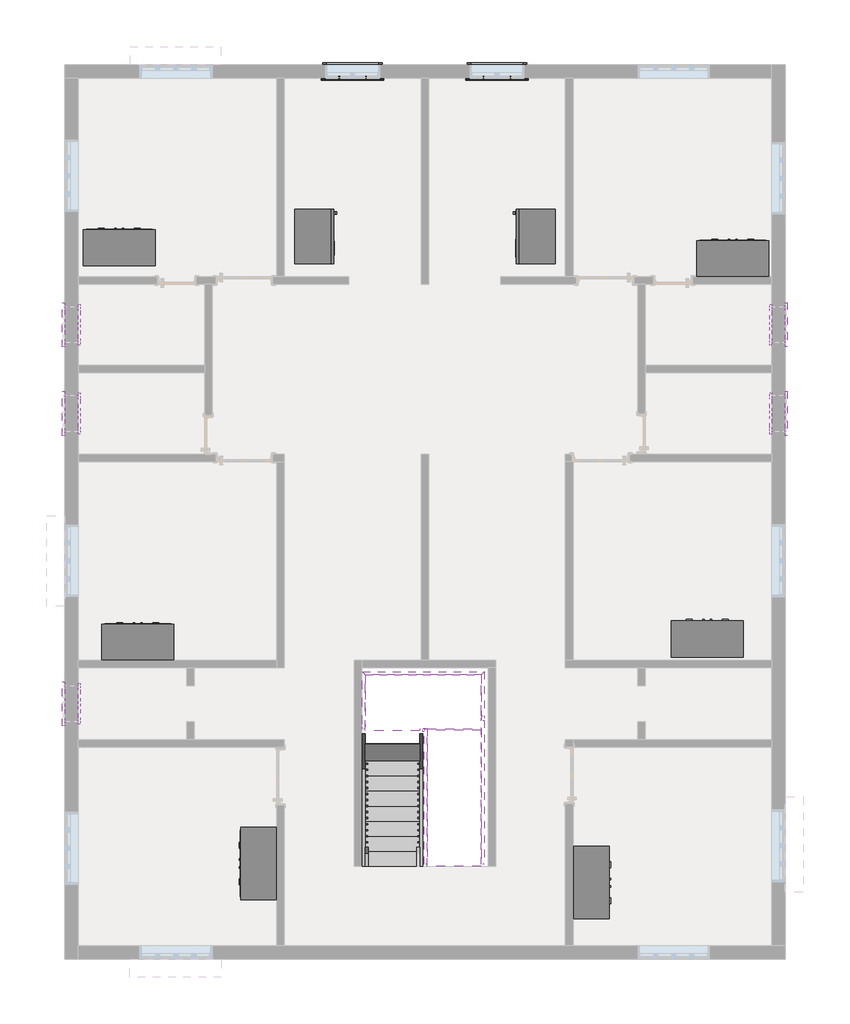
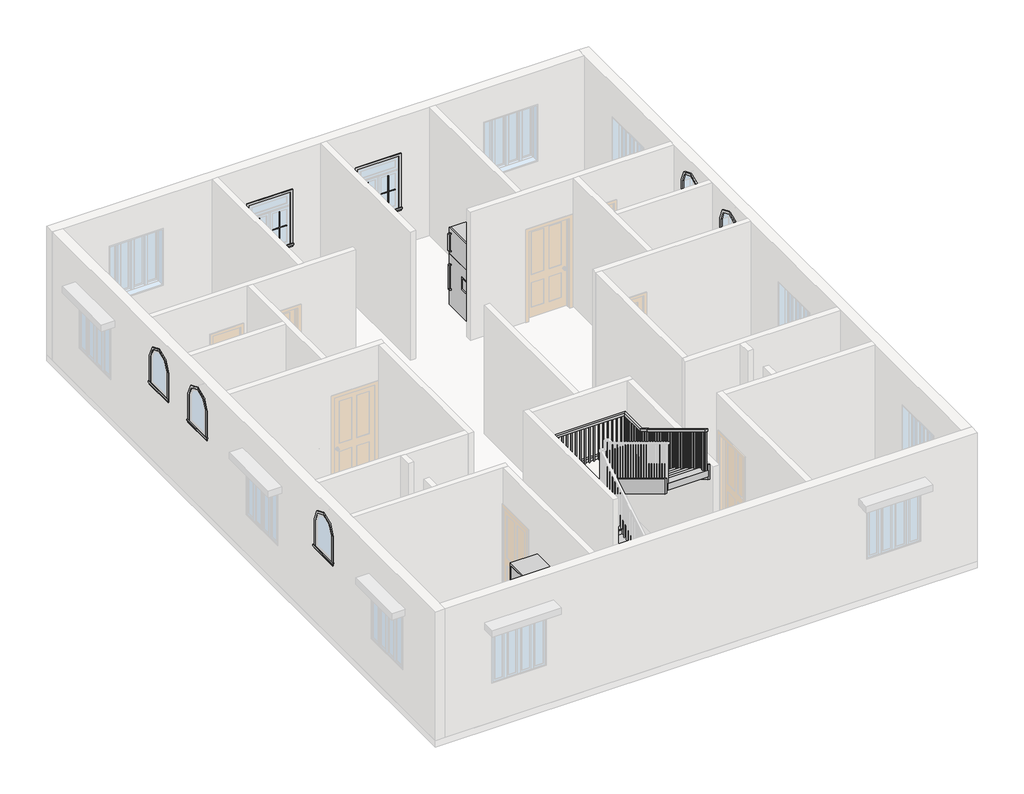
# One storey, part 3 of 4: 18 proxies, 8 furniture elements, 8 members, 2 stair flights, 1 railing, 1 slab.
"""IFC4 building model written with IfcOpenShell, lengths in millimetres."""

from ifc_helpers import new_model, si_unit, frame, origin, place, context, project, spatial, polyline, outline, extrude, faceted_brep, transform, mapped, element, save
from components import muntin_pattern_2x2_muntin_pattern_2x2_d1c6e638, muntin_pattern_2x2_muntin_pattern_2x2_37b95fb2, trim_window_exterior_flat_with_sill_80371c4b, trim_window_exterior_flat_arch_top_tree_centered_with_sill_b3d54518, trim_window_interior_flat_picture_frame_c1dcbb6d, trim_window_interior_flat_arch_top_tree_centered_picture_1d59b3d4, furniture_65fa61b5, furniture_3f4f9d7a, furniture_82e269c4, non_monolithic_landing_0f5a95a9, stair_flight_63be9a33, stair_flight_b6fb1fe0

model = new_model("IFC4")

# Units and contexts
model_context = context("Model", 3, world=origin())
ifc_project = project(units=[si_unit("LENGTHUNIT", "METRE", prefix="MILLI")], contexts=[model_context])

# Site, building, storey
site = spatial("IfcSite", under=ifc_project)
building = spatial("IfcBuilding", under=site)
storey = spatial("IfcBuildingStorey", under=building, Elevation=3352.8)

# Proxies
placement = place(None, origin())
muntin_pattern_2x2_muntin_pattern_2x2_shape = muntin_pattern_2x2_muntin_pattern_2x2_d1c6e638(model_context)
element("IfcBuildingElementProxy", 1, Name="Muntin Pattern_2x2 : Muntin Pattern_2x2", ObjectType="Muntin Pattern_2x2 : Muntin Pattern_2x2", at=placement, inside=storey, context=model_context, shape_type="MappedRepresentation", body=[
    mapped(muntin_pattern_2x2_muntin_pattern_2x2_shape, transform((-10531.1646954, 8361.6522103, 4337.05), x_axis=(-1.0, 0.0, 0.0), y_axis=(0.0, -1.0, 0.0), z_axis=(0.0, 0.0, 1.0))),
])
element("IfcBuildingElementProxy", 2, Name="Muntin Pattern_2x2 : Muntin Pattern_2x2", ObjectType="Muntin Pattern_2x2 : Muntin Pattern_2x2", at=placement, inside=storey, context=model_context, shape_type="MappedRepresentation", body=[
    mapped(muntin_pattern_2x2_muntin_pattern_2x2_shape, transform((-8092.7646954, 8361.6522103, 4337.05), x_axis=(-1.0, 0.0, 0.0), y_axis=(0.0, -1.0, 0.0), z_axis=(0.0, 0.0, 1.0))),
])
muntin_pattern_2x2_muntin_pattern_2x2_2_shape = muntin_pattern_2x2_muntin_pattern_2x2_37b95fb2(model_context)
element("IfcBuildingElementProxy", 3, Name="Muntin Pattern_2x2 : Muntin Pattern_2x2", ObjectType="Muntin Pattern_2x2 : Muntin Pattern_2x2", at=placement, inside=storey, context=model_context, shape_type="MappedRepresentation", body=[
    mapped(muntin_pattern_2x2_muntin_pattern_2x2_2_shape, transform((-10985.1896954, 8361.6522103, 4337.05), x_axis=(1.0, 0.0, 0.0), y_axis=(0.0, 1.0, 0.0), z_axis=(0.0, 0.0, 1.0))),
])
element("IfcBuildingElementProxy", 4, Name="Muntin Pattern_2x2 : Muntin Pattern_2x2", ObjectType="Muntin Pattern_2x2 : Muntin Pattern_2x2", at=placement, inside=storey, context=model_context, shape_type="MappedRepresentation", body=[
    mapped(muntin_pattern_2x2_muntin_pattern_2x2_2_shape, transform((-8546.7896954, 8361.6522103, 4337.05), x_axis=(1.0, 0.0, 0.0), y_axis=(0.0, 1.0, 0.0), z_axis=(0.0, 0.0, 1.0))),
])
trim_window_exterior_flat_with_sill_shape = trim_window_exterior_flat_with_sill_80371c4b(model_context)
element("IfcBuildingElementProxy", 5, Name="Trim-Window-Exterior-Flat : with Sill", ObjectType="Trim-Window-Exterior-Flat : with Sill", at=placement, inside=storey, context=model_context, shape_type="MappedRepresentation", body=[
    mapped(trim_window_exterior_flat_with_sill_shape, transform((-10758.1771954, 8352.1272103, 5486.4), x_axis=(-1.0, 0.0, 0.0), y_axis=(0.0, 0.0, -1.0), z_axis=(0.0, -1.0, 0.0))),
])
element("IfcBuildingElementProxy", 6, Name="Trim-Window-Exterior-Flat : with Sill", ObjectType="Trim-Window-Exterior-Flat : with Sill", at=placement, inside=storey, context=model_context, shape_type="MappedRepresentation", body=[
    mapped(trim_window_exterior_flat_with_sill_shape, transform((-8319.7771954, 8352.1272103, 5486.4), x_axis=(-1.0, 0.0, 0.0), y_axis=(0.0, 0.0, -1.0), z_axis=(0.0, -1.0, 0.0))),
])
trim_window_exterior_flat_arch_top_tree_centered_with_sill_shape = trim_window_exterior_flat_arch_top_tree_centered_with_sill_b3d54518(model_context)
element("IfcBuildingElementProxy", 7, Name="Trim-Window-Exterior-Flat-Arch-Top-Tree_Centered : with Sill", ObjectType="Trim-Window-Exterior-Flat-Arch-Top-Tree_Centered : with Sill", at=placement, inside=storey, context=model_context, shape_type="MappedRepresentation", body=[
    mapped(trim_window_exterior_flat_arch_top_tree_centered_with_sill_shape, transform((-15623.8646954, -2214.2727897, 6096.0), x_axis=(0.0, -1.0, 0.0), y_axis=(0.0, 0.0, 1.0), z_axis=(-1.0, 0.0, 0.0))),
])
element("IfcBuildingElementProxy", 8, Name="Trim-Window-Exterior-Flat-Arch-Top-Tree_Centered : with Sill", ObjectType="Trim-Window-Exterior-Flat-Arch-Top-Tree_Centered : with Sill", at=placement, inside=storey, context=model_context, shape_type="MappedRepresentation", body=[
    mapped(trim_window_exterior_flat_arch_top_tree_centered_with_sill_shape, transform((-3455.6771954, 2688.1919086, 6096.0), x_axis=(0.0, 1.0, 0.0), y_axis=(0.0, 0.0, 1.0), z_axis=(1.0, 0.0, 0.0))),
])
element("IfcBuildingElementProxy", 9, Name="Trim-Window-Exterior-Flat-Arch-Top-Tree_Centered : with Sill", ObjectType="Trim-Window-Exterior-Flat-Arch-Top-Tree_Centered : with Sill", at=placement, inside=storey, context=model_context, shape_type="MappedRepresentation", body=[
    mapped(trim_window_exterior_flat_arch_top_tree_centered_with_sill_shape, transform((-3455.6771954, 4186.5272103, 6096.0), x_axis=(0.0, 1.0, 0.0), y_axis=(0.0, 0.0, 1.0), z_axis=(1.0, 0.0, 0.0))),
])
element("IfcBuildingElementProxy", 10, Name="Trim-Window-Exterior-Flat-Arch-Top-Tree_Centered : with Sill", ObjectType="Trim-Window-Exterior-Flat-Arch-Top-Tree_Centered : with Sill", at=placement, inside=storey, context=model_context, shape_type="MappedRepresentation", body=[
    mapped(trim_window_exterior_flat_arch_top_tree_centered_with_sill_shape, transform((-15623.8646954, 2688.1919086, 6096.0), x_axis=(0.0, -1.0, 0.0), y_axis=(0.0, 0.0, 1.0), z_axis=(-1.0, 0.0, 0.0))),
])
element("IfcBuildingElementProxy", 11, Name="Trim-Window-Exterior-Flat-Arch-Top-Tree_Centered : with Sill", ObjectType="Trim-Window-Exterior-Flat-Arch-Top-Tree_Centered : with Sill", at=placement, inside=storey, context=model_context, shape_type="MappedRepresentation", body=[
    mapped(trim_window_exterior_flat_arch_top_tree_centered_with_sill_shape, transform((-15623.8646954, 4186.5272103, 6096.0), x_axis=(0.0, -1.0, 0.0), y_axis=(0.0, 0.0, 1.0), z_axis=(-1.0, 0.0, 0.0))),
])
trim_window_interior_flat_picture_frame_shape = trim_window_interior_flat_picture_frame_c1dcbb6d(model_context)
element("IfcBuildingElementProxy", 12, Name="Trim-Window-Interior-Flat : Picture Frame", ObjectType="Trim-Window-Interior-Flat : Picture Frame", at=placement, inside=storey, context=model_context, shape_type="MappedRepresentation", body=[
    mapped(trim_window_interior_flat_picture_frame_shape, transform((-10758.1771954, 8580.7272103, 5486.4), x_axis=(1.0, 0.0, 0.0), y_axis=(0.0, 0.0, -1.0), z_axis=(0.0, 1.0, 0.0))),
])
element("IfcBuildingElementProxy", 13, Name="Trim-Window-Interior-Flat : Picture Frame", ObjectType="Trim-Window-Interior-Flat : Picture Frame", at=placement, inside=storey, context=model_context, shape_type="MappedRepresentation", body=[
    mapped(trim_window_interior_flat_picture_frame_shape, transform((-8319.7771954, 8580.7272103, 5486.4), x_axis=(1.0, 0.0, 0.0), y_axis=(0.0, 0.0, -1.0), z_axis=(0.0, 1.0, 0.0))),
])
trim_window_interior_flat_arch_top_tree_centered_picture_shape = trim_window_interior_flat_arch_top_tree_centered_picture_1d59b3d4(model_context)
element("IfcBuildingElementProxy", 14, Name="Trim-Window-Interior-Flat-Arch-Top-Tree_Centered : Picture Frame", ObjectType="Trim-Window-Interior-Flat-Arch-Top-Tree_Centered : Picture Frame", at=placement, inside=storey, context=model_context, shape_type="MappedRepresentation", body=[
    mapped(trim_window_interior_flat_arch_top_tree_centered_picture_shape, transform((-15395.2646954, -2214.2727897, 6096.0), x_axis=(0.0, 1.0, 0.0), y_axis=(0.0, 0.0, 1.0), z_axis=(1.0, 0.0, 0.0))),
])
element("IfcBuildingElementProxy", 15, Name="Trim-Window-Interior-Flat-Arch-Top-Tree_Centered : Picture Frame", ObjectType="Trim-Window-Interior-Flat-Arch-Top-Tree_Centered : Picture Frame", at=placement, inside=storey, context=model_context, shape_type="MappedRepresentation", body=[
    mapped(trim_window_interior_flat_arch_top_tree_centered_picture_shape, transform((-3684.2771954, 2688.1919086, 6096.0), x_axis=(0.0, -1.0, 0.0), y_axis=(0.0, 0.0, 1.0), z_axis=(-1.0, 0.0, 0.0))),
])
element("IfcBuildingElementProxy", 16, Name="Trim-Window-Interior-Flat-Arch-Top-Tree_Centered : Picture Frame", ObjectType="Trim-Window-Interior-Flat-Arch-Top-Tree_Centered : Picture Frame", at=placement, inside=storey, context=model_context, shape_type="MappedRepresentation", body=[
    mapped(trim_window_interior_flat_arch_top_tree_centered_picture_shape, transform((-3684.2771954, 4186.5272103, 6096.0), x_axis=(0.0, -1.0, 0.0), y_axis=(0.0, 0.0, 1.0), z_axis=(-1.0, 0.0, 0.0))),
])
element("IfcBuildingElementProxy", 17, Name="Trim-Window-Interior-Flat-Arch-Top-Tree_Centered : Picture Frame", ObjectType="Trim-Window-Interior-Flat-Arch-Top-Tree_Centered : Picture Frame", at=placement, inside=storey, context=model_context, shape_type="MappedRepresentation", body=[
    mapped(trim_window_interior_flat_arch_top_tree_centered_picture_shape, transform((-15395.2646954, 2688.1919086, 6096.0), x_axis=(0.0, 1.0, 0.0), y_axis=(0.0, 0.0, 1.0), z_axis=(1.0, 0.0, 0.0))),
])
element("IfcBuildingElementProxy", 18, Name="Trim-Window-Interior-Flat-Arch-Top-Tree_Centered : Picture Frame", ObjectType="Trim-Window-Interior-Flat-Arch-Top-Tree_Centered : Picture Frame", at=placement, inside=storey, context=model_context, shape_type="MappedRepresentation", body=[
    mapped(trim_window_interior_flat_arch_top_tree_centered_picture_shape, transform((-15395.2646954, 4186.5272103, 6096.0), x_axis=(0.0, 1.0, 0.0), y_axis=(0.0, 0.0, 1.0), z_axis=(1.0, 0.0, 0.0))),
])

# Furniture
furniture_shape = furniture_65fa61b5(model_context)
element("IfcFurniture", 19, at=placement, inside=storey, context=model_context, shape_type="MappedRepresentation", body=[
    mapped(furniture_shape, transform((-11740.80602, 6289.078474, 3352.8), x_axis=(0.0, 1.0, 0.0), y_axis=(-1.0, 0.0, 0.0), z_axis=(0.0, 0.0, 1.0))),
])
furniture_2_shape = furniture_3f4f9d7a(model_context)
element("IfcFurniture", 20, at=placement, inside=storey, context=model_context, shape_type="MappedRepresentation", body=[
    mapped(furniture_2_shape, transform((-7338.7358708, 6289.078474, 3352.8), x_axis=(0.0, 1.0, 0.0), y_axis=(-1.0, 0.0, 0.0), z_axis=(0.0, 0.0, 1.0))),
])
furniture_3_shape = furniture_82e269c4(model_context)
element("IfcFurniture", 21, ObjectType="Wardrobe : 48\" x 72\" x 24\"", at=placement, inside=storey, context=model_context, shape_type="MappedRepresentation", body=[
    mapped(furniture_3_shape, transform((-14969.1544857, 4905.0525787, 3352.8), x_axis=(-1.0, 0.0, 0.0), y_axis=(0.0, -1.0, 0.0), z_axis=(0.0, 0.0, 1.0))),
])
element("IfcFurniture", 22, ObjectType="Wardrobe : 48\" x 72\" x 24\"", at=placement, inside=storey, context=model_context, shape_type="MappedRepresentation", body=[
    mapped(furniture_3_shape, transform((-4609.4240791, 4720.3884008, 3352.8), x_axis=(-1.0, 0.0, 0.0), y_axis=(0.0, -1.0, 0.0), z_axis=(0.0, 0.0, 1.0))),
])
element("IfcFurniture", 23, ObjectType="Wardrobe : 48\" x 72\" x 24\"", at=placement, inside=storey, context=model_context, shape_type="MappedRepresentation", body=[
    mapped(furniture_3_shape, transform((-14654.9354475, -1756.6115992, 3352.8), x_axis=(-1.0, 0.0, 0.0), y_axis=(0.0, -1.0, 0.0), z_axis=(0.0, 0.0, 1.0))),
])
element("IfcFurniture", 24, ObjectType="Wardrobe : 48\" x 72\" x 24\"", at=placement, inside=storey, context=model_context, shape_type="MappedRepresentation", body=[
    mapped(furniture_3_shape, transform((-5037.6875981, -1704.33178, 3352.8), x_axis=(-1.0, 0.0, 0.0), y_axis=(0.0, -1.0, 0.0), z_axis=(0.0, 0.0, 1.0))),
])
element("IfcFurniture", 25, ObjectType="Wardrobe : 48\" x 72\" x 24\"", at=placement, inside=storey, context=model_context, shape_type="MappedRepresentation", body=[
    mapped(furniture_3_shape, transform((-7316.016005, -4965.0574511, 3352.8), x_axis=(0.0, 1.0, 0.0), y_axis=(-1.0, 0.0, 0.0), z_axis=(0.0, 0.0, 1.0))),
])
element("IfcFurniture", 26, ObjectType="Wardrobe : 48\" x 72\" x 24\"", at=placement, inside=storey, context=model_context, shape_type="MappedRepresentation", body=[
    mapped(furniture_3_shape, transform((-11761.9383858, -5181.4279362, 3352.8), x_axis=(0.0, -1.0, 0.0), y_axis=(1.0, 0.0, 0.0), z_axis=(0.0, 0.0, 1.0))),
])

# Members
element("IfcMember", 27, ObjectType="Stringer - 2\" Width", at=placement, inside=storey, context=model_context, shape_type="SweptSolid", body=[
    extrude(outline(polyline([(-4957.4727897, 3352.8), (-4957.4727897, 3564.3517384), (-2643.0590204, 4953.0), (-2558.6343079, 4648.2), (-4717.6343079, 3352.8), (-4957.4727897, 3352.8)])), frame((-10593.0771954, 0.0, 0.0), z_axis=(1.0, 0.0, 0.0), x_axis=(0.0, 1.0, 0.0)), (0.0, 0.0, 1.0), 50.8),
])
element("IfcMember", 28, ObjectType="Stringer - 2\" Width", at=placement, inside=storey, context=model_context, shape_type="SweptSolid", body=[
    extrude(outline(polyline([(-4957.4727897, 3352.8), (-4957.4727897, 3564.3517384), (-2643.0590204, 4953.0), (-2639.7227897, 4953.0), (-2639.7227897, 4599.5469109), (-4717.6343079, 3352.8), (-4957.4727897, 3352.8)])), frame((-9627.8771954, 0.0, 0.0), z_axis=(1.0, 0.0, 0.0), x_axis=(0.0, 1.0, 0.0)), (0.0, 0.0, 1.0), 50.8),
])
element("IfcMember", 29, ObjectType="Stringer - 2\" Width", at=placement, inside=storey, context=model_context, shape_type="SweptSolid", body=[
    extrude(outline(polyline([(-2414.1365589, 4953.0), (-2498.5612714, 4648.2), (-4925.7227897, 6104.4969109), (-4925.7227897, 6459.9517384), (-2414.1365589, 4953.0)])), frame((-8586.4771954, 0.0, 0.0), z_axis=(1.0, 0.0, 0.0), x_axis=(0.0, 1.0, 0.0)), (0.0, 0.0, 1.0), 50.8),
])
element("IfcMember", 30, ObjectType="Stringer - 2\" Width", at=placement, inside=storey, context=model_context, shape_type="SweptSolid", body=[
    extrude(outline(polyline([(-2639.7227897, 5088.3517384), (-2639.7227897, 4732.8969109), (-4925.7227897, 6104.4969109), (-4925.7227897, 6459.9517384), (-2639.7227897, 5088.3517384)])), frame((-9551.6771954, 0.0, 0.0), z_axis=(1.0, 0.0, 0.0), x_axis=(0.0, 1.0, 0.0)), (0.0, 0.0, 1.0), 50.8),
])
element("IfcMember", 31, ObjectType="Stringer - 2\" Width", at=placement, inside=storey, context=model_context, shape_type="Brep", body=[
    faceted_brep([(-8586.4771954, -2414.1365589, 4953.0), (-8535.6771954, -2414.1365589, 4953.0), (-8535.6771954, -1674.5227897, 4953.0), (-8586.4771954, -1725.3227897, 4953.0), (-8586.4771954, -2498.5612714, 4648.2), (-8586.4771954, -1725.3227897, 4648.2), (-8535.6771954, -2498.5612714, 4648.2), (-8535.6771954, -1674.5227897, 4648.2)], [[[0, 1, 2, 3]], [[4, 0, 3, 5]], [[6, 4, 5, 7]], [[1, 6, 7, 2]], [[1, 0, 4, 6]], [[2, 7, 5, 3]]]),
])
element("IfcMember", 32, ObjectType="Stringer - 2\" Width", at=placement, inside=storey, context=model_context, shape_type="SweptSolid", body=[
    extrude(outline(polyline([(-8535.6771954, -1674.5227897), (-8586.4771954, -1725.3227897), (-10542.2771954, -1725.3227897), (-10593.0771954, -1674.5227897), (-8535.6771954, -1674.5227897)])), frame((0.0, 0.0, 4648.2), z_axis=(0.0, 0.0, 1.0), x_axis=(1.0, 0.0, 0.0)), (0.0, 0.0, 1.0), 304.8),
])
element("IfcMember", 33, ObjectType="Stringer - 2\" Width", at=placement, inside=storey, context=model_context, shape_type="Brep", body=[
    faceted_brep([(-10542.2771954, -1725.3227897, 4953.0), (-10593.0771954, -1674.5227897, 4953.0), (-10593.0771954, -2643.0590204, 4953.0), (-10542.2771954, -2643.0590204, 4953.0), (-10542.2771954, -1725.3227897, 4648.2), (-10542.2771954, -2558.6343079, 4648.2), (-10593.0771954, -1674.5227897, 4648.2), (-10593.0771954, -2558.6343079, 4648.2)], [[[0, 1, 2, 3]], [[4, 0, 3, 5]], [[6, 4, 5, 7]], [[1, 6, 7, 2]], [[1, 0, 4, 6]], [[2, 7, 5, 3]]]),
])
element("IfcMember", 34, ObjectType="Stringer - 2\" Width", at=placement, inside=storey, context=model_context, shape_type="SweptSolid", body=[
    extrude(outline(polyline([(-9577.0771954, -2690.5227897), (-9577.0771954, -2639.7227897), (-9551.6771954, -2639.7227897), (-9551.6771954, -2690.5227897), (-9577.0771954, -2690.5227897)])), frame((0.0, 0.0, 4648.2), z_axis=(0.0, 0.0, 1.0), x_axis=(1.0, 0.0, 0.0)), (0.0, 0.0, 1.0), 304.8),
])

# Railing
element("IfcRailing", 35, ObjectType="Handrail - Rectangular", at=placement, inside=storey, context=model_context, shape_type="SolidModel", body=[
    faceted_brep([(-10542.2771954, -4957.4727897, 4419.6), (-10542.2771954, -4957.4727897, 4360.3575287), (-10491.4771954, -4957.4727897, 4360.3575287), (-10491.4771954, -4957.4727897, 4419.6), (-10542.2771954, -2671.4727897, 5791.2), (-10542.2771954, -2657.4020042, 5740.4), (-10491.4771954, -2657.4020042, 5740.4), (-10491.4771954, -2671.4727897, 5791.2), (-10542.2771954, -1725.3227897, 5791.2), (-10542.2771954, -1725.3227897, 5740.4), (-10491.4771954, -1776.1227897, 5740.4), (-10491.4771954, -1776.1227897, 5791.2), (-8586.4771954, -1725.3227897, 5791.2), (-8586.4771954, -1725.3227897, 5740.4), (-8637.2771954, -1776.1227897, 5740.4), (-8637.2771954, -1776.1227897, 5791.2), (-8586.4771954, -2385.7227897, 5791.2), (-8586.4771954, -2399.7935751, 5740.4), (-8637.2771954, -2399.7935751, 5740.4), (-8637.2771954, -2385.7227897, 5791.2), (-8586.4771954, -2639.7227897, 5943.6), (-8586.4771954, -2665.859174, 5900.0393594), (-8637.2771954, -2665.859174, 5900.0393594), (-8637.2771954, -2639.7227897, 5943.6), (-8586.4771954, -4925.7227897, 7315.2), (-8637.2771954, -4925.7227897, 7315.2), (-8637.2771954, -4925.7227897, 7255.9575287), (-8586.4771954, -4925.7227897, 7255.9575287)], [[[0, 1, 2, 3]], [[1, 0, 4, 5]], [[2, 1, 5, 6]], [[3, 2, 6, 7]], [[0, 3, 7, 4]], [[5, 4, 8, 9]], [[6, 5, 9, 10]], [[7, 6, 10, 11]], [[4, 7, 11, 8]], [[9, 8, 12, 13]], [[10, 9, 13, 14]], [[11, 10, 14, 15]], [[8, 11, 15, 12]], [[13, 12, 16, 17]], [[14, 13, 17, 18]], [[15, 14, 18, 19]], [[12, 15, 19, 16]], [[17, 16, 20, 21]], [[18, 17, 21, 22]], [[19, 18, 22, 23]], [[16, 19, 23, 20]], [[24, 25, 26, 27]], [[21, 20, 24, 27]], [[22, 21, 27, 26]], [[23, 22, 26, 25]], [[20, 23, 25, 24]]]),
    extrude(outline(polyline([(-4865.3977897, 7219.7625287), (-4865.3977897, 6248.4), (-4884.4477897, 6248.4), (-4884.4477897, 7231.1925287), (-4865.3977897, 7219.7625287)])), frame((-8621.4021954, 0.0, 0.0), z_axis=(1.0, 0.0, 0.0), x_axis=(0.0, 1.0, 0.0)), (0.0, 0.0, 1.0), 19.05),
    extrude(outline(polyline([(-4763.7977897, 7158.8025287), (-4763.7977897, 6248.4), (-4782.8477897, 6248.4), (-4782.8477897, 7170.2325287), (-4763.7977897, 7158.8025287)])), frame((-8621.4021954, 0.0, 0.0), z_axis=(1.0, 0.0, 0.0), x_axis=(0.0, 1.0, 0.0)), (0.0, 0.0, 1.0), 19.05),
    extrude(outline(polyline([(-4662.1977897, 7097.8425287), (-4662.1977897, 6248.4), (-4681.2477897, 6248.4), (-4681.2477897, 7109.2725287), (-4662.1977897, 7097.8425287)])), frame((-8621.4021954, 0.0, 0.0), z_axis=(1.0, 0.0, 0.0), x_axis=(0.0, 1.0, 0.0)), (0.0, 0.0, 1.0), 19.05),
    extrude(outline(polyline([(-4560.5977897, 7036.8825287), (-4560.5977897, 6096.0), (-4579.6477897, 6096.0), (-4579.6477897, 7048.3125287), (-4560.5977897, 7036.8825287)])), frame((-8621.4021954, 0.0, 0.0), z_axis=(1.0, 0.0, 0.0), x_axis=(0.0, 1.0, 0.0)), (0.0, 0.0, 1.0), 19.05),
    extrude(outline(polyline([(-4458.9977897, 6975.9225287), (-4458.9977897, 6096.0), (-4478.0477897, 6096.0), (-4478.0477897, 6987.3525287), (-4458.9977897, 6975.9225287)])), frame((-8621.4021954, 0.0, 0.0), z_axis=(1.0, 0.0, 0.0), x_axis=(0.0, 1.0, 0.0)), (0.0, 0.0, 1.0), 19.05),
    extrude(outline(polyline([(-4357.3977897, 6914.9625287), (-4357.3977897, 5943.6), (-4376.4477897, 5943.6), (-4376.4477897, 6926.3925287), (-4357.3977897, 6914.9625287)])), frame((-8621.4021954, 0.0, 0.0), z_axis=(1.0, 0.0, 0.0), x_axis=(0.0, 1.0, 0.0)), (0.0, 0.0, 1.0), 19.05),
    extrude(outline(polyline([(-4255.7977897, 6854.0025287), (-4255.7977897, 5943.6), (-4274.8477897, 5943.6), (-4274.8477897, 6865.4325287), (-4255.7977897, 6854.0025287)])), frame((-8621.4021954, 0.0, 0.0), z_axis=(1.0, 0.0, 0.0), x_axis=(0.0, 1.0, 0.0)), (0.0, 0.0, 1.0), 19.05),
    extrude(outline(polyline([(-4154.1977897, 6793.0425287), (-4154.1977897, 5943.6), (-4173.2477897, 5943.6), (-4173.2477897, 6804.4725287), (-4154.1977897, 6793.0425287)])), frame((-8621.4021954, 0.0, 0.0), z_axis=(1.0, 0.0, 0.0), x_axis=(0.0, 1.0, 0.0)), (0.0, 0.0, 1.0), 19.05),
    extrude(outline(polyline([(-4052.5977897, 6732.0825287), (-4052.5977897, 5791.2), (-4071.6477897, 5791.2), (-4071.6477897, 6743.5125287), (-4052.5977897, 6732.0825287)])), frame((-8621.4021954, 0.0, 0.0), z_axis=(1.0, 0.0, 0.0), x_axis=(0.0, 1.0, 0.0)), (0.0, 0.0, 1.0), 19.05),
    extrude(outline(polyline([(-3950.9977897, 6671.1225287), (-3950.9977897, 5791.2), (-3970.0477897, 5791.2), (-3970.0477897, 6682.5525287), (-3950.9977897, 6671.1225287)])), frame((-8621.4021954, 0.0, 0.0), z_axis=(1.0, 0.0, 0.0), x_axis=(0.0, 1.0, 0.0)), (0.0, 0.0, 1.0), 19.05),
    extrude(outline(polyline([(-3849.3977897, 6610.1625287), (-3849.3977897, 5638.8), (-3868.4477897, 5638.8), (-3868.4477897, 6621.5925287), (-3849.3977897, 6610.1625287)])), frame((-8621.4021954, 0.0, 0.0), z_axis=(1.0, 0.0, 0.0), x_axis=(0.0, 1.0, 0.0)), (0.0, 0.0, 1.0), 19.05),
    extrude(outline(polyline([(-3747.7977897, 6549.2025287), (-3747.7977897, 5638.8), (-3766.8477897, 5638.8), (-3766.8477897, 6560.6325287), (-3747.7977897, 6549.2025287)])), frame((-8621.4021954, 0.0, 0.0), z_axis=(1.0, 0.0, 0.0), x_axis=(0.0, 1.0, 0.0)), (0.0, 0.0, 1.0), 19.05),
    extrude(outline(polyline([(-3646.1977897, 6488.2425287), (-3646.1977897, 5638.8), (-3665.2477897, 5638.8), (-3665.2477897, 6499.6725287), (-3646.1977897, 6488.2425287)])), frame((-8621.4021954, 0.0, 0.0), z_axis=(1.0, 0.0, 0.0), x_axis=(0.0, 1.0, 0.0)), (0.0, 0.0, 1.0), 19.05),
    extrude(outline(polyline([(-3544.5977897, 6427.2825287), (-3544.5977897, 5486.4), (-3563.6477897, 5486.4), (-3563.6477897, 6438.7125287), (-3544.5977897, 6427.2825287)])), frame((-8621.4021954, 0.0, 0.0), z_axis=(1.0, 0.0, 0.0), x_axis=(0.0, 1.0, 0.0)), (0.0, 0.0, 1.0), 19.05),
    extrude(outline(polyline([(-3442.9977897, 6366.3225287), (-3442.9977897, 5486.4), (-3462.0477897, 5486.4), (-3462.0477897, 6377.7525287), (-3442.9977897, 6366.3225287)])), frame((-8621.4021954, 0.0, 0.0), z_axis=(1.0, 0.0, 0.0), x_axis=(0.0, 1.0, 0.0)), (0.0, 0.0, 1.0), 19.05),
    extrude(outline(polyline([(-3341.3977897, 6305.3625287), (-3341.3977897, 5334.0), (-3360.4477897, 5334.0), (-3360.4477897, 6316.7925287), (-3341.3977897, 6305.3625287)])), frame((-8621.4021954, 0.0, 0.0), z_axis=(1.0, 0.0, 0.0), x_axis=(0.0, 1.0, 0.0)), (0.0, 0.0, 1.0), 19.05),
    extrude(outline(polyline([(-3239.7977897, 6244.4025287), (-3239.7977897, 5334.0), (-3258.8477897, 5334.0), (-3258.8477897, 6255.8325287), (-3239.7977897, 6244.4025287)])), frame((-8621.4021954, 0.0, 0.0), z_axis=(1.0, 0.0, 0.0), x_axis=(0.0, 1.0, 0.0)), (0.0, 0.0, 1.0), 19.05),
    extrude(outline(polyline([(-3138.1977897, 6183.4425287), (-3138.1977897, 5334.0), (-3157.2477897, 5334.0), (-3157.2477897, 6194.8725287), (-3138.1977897, 6183.4425287)])), frame((-8621.4021954, 0.0, 0.0), z_axis=(1.0, 0.0, 0.0), x_axis=(0.0, 1.0, 0.0)), (0.0, 0.0, 1.0), 19.05),
    extrude(outline(polyline([(-3036.5977897, 6122.4825287), (-3036.5977897, 5181.6), (-3055.6477897, 5181.6), (-3055.6477897, 6133.9125287), (-3036.5977897, 6122.4825287)])), frame((-8621.4021954, 0.0, 0.0), z_axis=(1.0, 0.0, 0.0), x_axis=(0.0, 1.0, 0.0)), (0.0, 0.0, 1.0), 19.05),
    extrude(outline(polyline([(-2934.9977897, 6061.5225287), (-2934.9977897, 5181.6), (-2954.0477897, 5181.6), (-2954.0477897, 6072.9525287), (-2934.9977897, 6061.5225287)])), frame((-8621.4021954, 0.0, 0.0), z_axis=(1.0, 0.0, 0.0), x_axis=(0.0, 1.0, 0.0)), (0.0, 0.0, 1.0), 19.05),
    extrude(outline(polyline([(-2833.3977897, 6000.5625287), (-2833.3977897, 5029.2), (-2852.4477897, 5029.2), (-2852.4477897, 6011.9925287), (-2833.3977897, 6000.5625287)])), frame((-8621.4021954, 0.0, 0.0), z_axis=(1.0, 0.0, 0.0), x_axis=(0.0, 1.0, 0.0)), (0.0, 0.0, 1.0), 19.05),
    extrude(outline(polyline([(-2731.7977897, 5939.6025287), (-2731.7977897, 5029.2), (-2750.8477897, 5029.2), (-2750.8477897, 5951.0325287), (-2731.7977897, 5939.6025287)])), frame((-8621.4021954, 0.0, 0.0), z_axis=(1.0, 0.0, 0.0), x_axis=(0.0, 1.0, 0.0)), (0.0, 0.0, 1.0), 19.05),
    extrude(outline(polyline([(-2553.9977897, 5832.9225287), (-2553.9977897, 4876.8), (-2573.0477897, 4876.8), (-2573.0477897, 5844.3525287), (-2553.9977897, 5832.9225287)])), frame((-8621.4021954, 0.0, 0.0), z_axis=(1.0, 0.0, 0.0), x_axis=(0.0, 1.0, 0.0)), (0.0, 0.0, 1.0), 19.05),
    extrude(outline(polyline([(-2452.3977897, 5771.9625287), (-2452.3977897, 4876.8), (-2471.4477897, 4876.8), (-2471.4477897, 5783.3925287), (-2452.3977897, 5771.9625287)])), frame((-8621.4021954, 0.0, 0.0), z_axis=(1.0, 0.0, 0.0), x_axis=(0.0, 1.0, 0.0)), (0.0, 0.0, 1.0), 19.05),
    extrude(outline(polyline([(-8602.3521954, -2350.7977897), (-8602.3521954, -2369.8477897), (-8621.4021954, -2369.8477897), (-8621.4021954, -2350.7977897), (-8602.3521954, -2350.7977897)])), frame((0.0, 0.0, 4876.8), z_axis=(0.0, 0.0, 1.0), x_axis=(1.0, 0.0, 0.0)), (0.0, 0.0, 1.0), 863.6),
    extrude(outline(polyline([(-8602.3521954, -2249.1977897), (-8602.3521954, -2268.2477897), (-8621.4021954, -2268.2477897), (-8621.4021954, -2249.1977897), (-8602.3521954, -2249.1977897)])), frame((0.0, 0.0, 4876.8), z_axis=(0.0, 0.0, 1.0), x_axis=(1.0, 0.0, 0.0)), (0.0, 0.0, 1.0), 863.6),
    extrude(outline(polyline([(-8602.3521954, -2147.5977897), (-8602.3521954, -2166.6477897), (-8621.4021954, -2166.6477897), (-8621.4021954, -2147.5977897), (-8602.3521954, -2147.5977897)])), frame((0.0, 0.0, 4876.8), z_axis=(0.0, 0.0, 1.0), x_axis=(1.0, 0.0, 0.0)), (0.0, 0.0, 1.0), 863.6),
    extrude(outline(polyline([(-8602.3521954, -2045.9977897), (-8602.3521954, -2065.0477897), (-8621.4021954, -2065.0477897), (-8621.4021954, -2045.9977897), (-8602.3521954, -2045.9977897)])), frame((0.0, 0.0, 4876.8), z_axis=(0.0, 0.0, 1.0), x_axis=(1.0, 0.0, 0.0)), (0.0, 0.0, 1.0), 863.6),
    extrude(outline(polyline([(-8602.3521954, -1944.3977897), (-8602.3521954, -1963.4477897), (-8621.4021954, -1963.4477897), (-8621.4021954, -1944.3977897), (-8602.3521954, -1944.3977897)])), frame((0.0, 0.0, 4876.8), z_axis=(0.0, 0.0, 1.0), x_axis=(1.0, 0.0, 0.0)), (0.0, 0.0, 1.0), 863.6),
    extrude(outline(polyline([(-8602.3521954, -1842.7977897), (-8602.3521954, -1861.8477897), (-8621.4021954, -1861.8477897), (-8621.4021954, -1842.7977897), (-8602.3521954, -1842.7977897)])), frame((0.0, 0.0, 4876.8), z_axis=(0.0, 0.0, 1.0), x_axis=(1.0, 0.0, 0.0)), (0.0, 0.0, 1.0), 863.6),
    extrude(outline(polyline([(-8697.6021954, -1741.1977897), (-8678.5521954, -1741.1977897), (-8678.5521954, -1760.2477897), (-8697.6021954, -1760.2477897), (-8697.6021954, -1741.1977897)])), frame((0.0, 0.0, 4876.8), z_axis=(0.0, 0.0, 1.0), x_axis=(1.0, 0.0, 0.0)), (0.0, 0.0, 1.0), 863.6),
    extrude(outline(polyline([(-8799.2021954, -1741.1977897), (-8780.1521954, -1741.1977897), (-8780.1521954, -1760.2477897), (-8799.2021954, -1760.2477897), (-8799.2021954, -1741.1977897)])), frame((0.0, 0.0, 4876.8), z_axis=(0.0, 0.0, 1.0), x_axis=(1.0, 0.0, 0.0)), (0.0, 0.0, 1.0), 863.6),
    extrude(outline(polyline([(-8900.8021954, -1741.1977897), (-8881.7521954, -1741.1977897), (-8881.7521954, -1760.2477897), (-8900.8021954, -1760.2477897), (-8900.8021954, -1741.1977897)])), frame((0.0, 0.0, 4876.8), z_axis=(0.0, 0.0, 1.0), x_axis=(1.0, 0.0, 0.0)), (0.0, 0.0, 1.0), 863.6),
    extrude(outline(polyline([(-9002.4021954, -1741.1977897), (-8983.3521954, -1741.1977897), (-8983.3521954, -1760.2477897), (-9002.4021954, -1760.2477897), (-9002.4021954, -1741.1977897)])), frame((0.0, 0.0, 4876.8), z_axis=(0.0, 0.0, 1.0), x_axis=(1.0, 0.0, 0.0)), (0.0, 0.0, 1.0), 863.6),
    extrude(outline(polyline([(-9104.0021954, -1741.1977897), (-9084.9521954, -1741.1977897), (-9084.9521954, -1760.2477897), (-9104.0021954, -1760.2477897), (-9104.0021954, -1741.1977897)])), frame((0.0, 0.0, 4876.8), z_axis=(0.0, 0.0, 1.0), x_axis=(1.0, 0.0, 0.0)), (0.0, 0.0, 1.0), 863.6),
    extrude(outline(polyline([(-9205.6021954, -1741.1977897), (-9186.5521954, -1741.1977897), (-9186.5521954, -1760.2477897), (-9205.6021954, -1760.2477897), (-9205.6021954, -1741.1977897)])), frame((0.0, 0.0, 4876.8), z_axis=(0.0, 0.0, 1.0), x_axis=(1.0, 0.0, 0.0)), (0.0, 0.0, 1.0), 863.6),
    extrude(outline(polyline([(-9307.2021954, -1741.1977897), (-9288.1521954, -1741.1977897), (-9288.1521954, -1760.2477897), (-9307.2021954, -1760.2477897), (-9307.2021954, -1741.1977897)])), frame((0.0, 0.0, 4876.8), z_axis=(0.0, 0.0, 1.0), x_axis=(1.0, 0.0, 0.0)), (0.0, 0.0, 1.0), 863.6),
    extrude(outline(polyline([(-9408.8021954, -1741.1977897), (-9389.7521954, -1741.1977897), (-9389.7521954, -1760.2477897), (-9408.8021954, -1760.2477897), (-9408.8021954, -1741.1977897)])), frame((0.0, 0.0, 4876.8), z_axis=(0.0, 0.0, 1.0), x_axis=(1.0, 0.0, 0.0)), (0.0, 0.0, 1.0), 863.6),
    extrude(outline(polyline([(-9510.4021954, -1741.1977897), (-9491.3521954, -1741.1977897), (-9491.3521954, -1760.2477897), (-9510.4021954, -1760.2477897), (-9510.4021954, -1741.1977897)])), frame((0.0, 0.0, 4876.8), z_axis=(0.0, 0.0, 1.0), x_axis=(1.0, 0.0, 0.0)), (0.0, 0.0, 1.0), 863.6),
    extrude(outline(polyline([(-9612.0021954, -1741.1977897), (-9592.9521954, -1741.1977897), (-9592.9521954, -1760.2477897), (-9612.0021954, -1760.2477897), (-9612.0021954, -1741.1977897)])), frame((0.0, 0.0, 4876.8), z_axis=(0.0, 0.0, 1.0), x_axis=(1.0, 0.0, 0.0)), (0.0, 0.0, 1.0), 863.6),
    extrude(outline(polyline([(-9713.6021954, -1741.1977897), (-9694.5521954, -1741.1977897), (-9694.5521954, -1760.2477897), (-9713.6021954, -1760.2477897), (-9713.6021954, -1741.1977897)])), frame((0.0, 0.0, 4876.8), z_axis=(0.0, 0.0, 1.0), x_axis=(1.0, 0.0, 0.0)), (0.0, 0.0, 1.0), 863.6),
    extrude(outline(polyline([(-9815.2021954, -1741.1977897), (-9796.1521954, -1741.1977897), (-9796.1521954, -1760.2477897), (-9815.2021954, -1760.2477897), (-9815.2021954, -1741.1977897)])), frame((0.0, 0.0, 4876.8), z_axis=(0.0, 0.0, 1.0), x_axis=(1.0, 0.0, 0.0)), (0.0, 0.0, 1.0), 863.6),
    extrude(outline(polyline([(-9916.8021954, -1741.1977897), (-9897.7521954, -1741.1977897), (-9897.7521954, -1760.2477897), (-9916.8021954, -1760.2477897), (-9916.8021954, -1741.1977897)])), frame((0.0, 0.0, 4876.8), z_axis=(0.0, 0.0, 1.0), x_axis=(1.0, 0.0, 0.0)), (0.0, 0.0, 1.0), 863.6),
    extrude(outline(polyline([(-10018.4021954, -1741.1977897), (-9999.3521954, -1741.1977897), (-9999.3521954, -1760.2477897), (-10018.4021954, -1760.2477897), (-10018.4021954, -1741.1977897)])), frame((0.0, 0.0, 4876.8), z_axis=(0.0, 0.0, 1.0), x_axis=(1.0, 0.0, 0.0)), (0.0, 0.0, 1.0), 863.6),
    extrude(outline(polyline([(-10120.0021954, -1741.1977897), (-10100.9521954, -1741.1977897), (-10100.9521954, -1760.2477897), (-10120.0021954, -1760.2477897), (-10120.0021954, -1741.1977897)])), frame((0.0, 0.0, 4876.8), z_axis=(0.0, 0.0, 1.0), x_axis=(1.0, 0.0, 0.0)), (0.0, 0.0, 1.0), 863.6),
    extrude(outline(polyline([(-10221.6021954, -1741.1977897), (-10202.5521954, -1741.1977897), (-10202.5521954, -1760.2477897), (-10221.6021954, -1760.2477897), (-10221.6021954, -1741.1977897)])), frame((0.0, 0.0, 4876.8), z_axis=(0.0, 0.0, 1.0), x_axis=(1.0, 0.0, 0.0)), (0.0, 0.0, 1.0), 863.6),
    extrude(outline(polyline([(-10323.2021954, -1741.1977897), (-10304.1521954, -1741.1977897), (-10304.1521954, -1760.2477897), (-10323.2021954, -1760.2477897), (-10323.2021954, -1741.1977897)])), frame((0.0, 0.0, 4876.8), z_axis=(0.0, 0.0, 1.0), x_axis=(1.0, 0.0, 0.0)), (0.0, 0.0, 1.0), 863.6),
    extrude(outline(polyline([(-10424.8021954, -1741.1977897), (-10405.7521954, -1741.1977897), (-10405.7521954, -1760.2477897), (-10424.8021954, -1760.2477897), (-10424.8021954, -1741.1977897)])), frame((0.0, 0.0, 4876.8), z_axis=(0.0, 0.0, 1.0), x_axis=(1.0, 0.0, 0.0)), (0.0, 0.0, 1.0), 863.6),
    extrude(outline(polyline([(-10526.4021954, -1766.5977897), (-10526.4021954, -1747.5477897), (-10507.3521954, -1747.5477897), (-10507.3521954, -1766.5977897), (-10526.4021954, -1766.5977897)])), frame((0.0, 0.0, 4876.8), z_axis=(0.0, 0.0, 1.0), x_axis=(1.0, 0.0, 0.0)), (0.0, 0.0, 1.0), 863.6),
    extrude(outline(polyline([(-10526.4021954, -1868.1977897), (-10526.4021954, -1849.1477897), (-10507.3521954, -1849.1477897), (-10507.3521954, -1868.1977897), (-10526.4021954, -1868.1977897)])), frame((0.0, 0.0, 4876.8), z_axis=(0.0, 0.0, 1.0), x_axis=(1.0, 0.0, 0.0)), (0.0, 0.0, 1.0), 863.6),
    extrude(outline(polyline([(-10526.4021954, -1969.7977897), (-10526.4021954, -1950.7477897), (-10507.3521954, -1950.7477897), (-10507.3521954, -1969.7977897), (-10526.4021954, -1969.7977897)])), frame((0.0, 0.0, 4876.8), z_axis=(0.0, 0.0, 1.0), x_axis=(1.0, 0.0, 0.0)), (0.0, 0.0, 1.0), 863.6),
    extrude(outline(polyline([(-10526.4021954, -2071.3977897), (-10526.4021954, -2052.3477897), (-10507.3521954, -2052.3477897), (-10507.3521954, -2071.3977897), (-10526.4021954, -2071.3977897)])), frame((0.0, 0.0, 4876.8), z_axis=(0.0, 0.0, 1.0), x_axis=(1.0, 0.0, 0.0)), (0.0, 0.0, 1.0), 863.6),
    extrude(outline(polyline([(-10526.4021954, -2172.9977897), (-10526.4021954, -2153.9477897), (-10507.3521954, -2153.9477897), (-10507.3521954, -2172.9977897), (-10526.4021954, -2172.9977897)])), frame((0.0, 0.0, 4876.8), z_axis=(0.0, 0.0, 1.0), x_axis=(1.0, 0.0, 0.0)), (0.0, 0.0, 1.0), 863.6),
    extrude(outline(polyline([(-10526.4021954, -2274.5977897), (-10526.4021954, -2255.5477897), (-10507.3521954, -2255.5477897), (-10507.3521954, -2274.5977897), (-10526.4021954, -2274.5977897)])), frame((0.0, 0.0, 4876.8), z_axis=(0.0, 0.0, 1.0), x_axis=(1.0, 0.0, 0.0)), (0.0, 0.0, 1.0), 863.6),
    extrude(outline(polyline([(-10526.4021954, -2376.1977897), (-10526.4021954, -2357.1477897), (-10507.3521954, -2357.1477897), (-10507.3521954, -2376.1977897), (-10526.4021954, -2376.1977897)])), frame((0.0, 0.0, 4876.8), z_axis=(0.0, 0.0, 1.0), x_axis=(1.0, 0.0, 0.0)), (0.0, 0.0, 1.0), 863.6),
    extrude(outline(polyline([(-10526.4021954, -2477.7977897), (-10526.4021954, -2458.7477897), (-10507.3521954, -2458.7477897), (-10507.3521954, -2477.7977897), (-10526.4021954, -2477.7977897)])), frame((0.0, 0.0, 4876.8), z_axis=(0.0, 0.0, 1.0), x_axis=(1.0, 0.0, 0.0)), (0.0, 0.0, 1.0), 863.6),
    extrude(outline(polyline([(-10526.4021954, -2579.3977897), (-10526.4021954, -2560.3477897), (-10507.3521954, -2560.3477897), (-10507.3521954, -2579.3977897), (-10526.4021954, -2579.3977897)])), frame((0.0, 0.0, 4876.8), z_axis=(0.0, 0.0, 1.0), x_axis=(1.0, 0.0, 0.0)), (0.0, 0.0, 1.0), 863.6),
    extrude(outline(polyline([(-2712.7477897, 5707.1925287), (-2712.7477897, 4724.4), (-2731.7977897, 4724.4), (-2731.7977897, 5695.7625287), (-2712.7477897, 5707.1925287)])), frame((-10526.4021954, 0.0, 0.0), z_axis=(1.0, 0.0, 0.0), x_axis=(0.0, 1.0, 0.0)), (0.0, 0.0, 1.0), 19.05),
    extrude(outline(polyline([(-2814.3477897, 5646.2325287), (-2814.3477897, 4724.4), (-2833.3977897, 4724.4), (-2833.3977897, 5634.8025287), (-2814.3477897, 5646.2325287)])), frame((-10526.4021954, 0.0, 0.0), z_axis=(1.0, 0.0, 0.0), x_axis=(0.0, 1.0, 0.0)), (0.0, 0.0, 1.0), 19.05),
    extrude(outline(polyline([(-2915.9477897, 5585.2725287), (-2915.9477897, 4724.4), (-2934.9977897, 4724.4), (-2934.9977897, 5573.8425287), (-2915.9477897, 5585.2725287)])), frame((-10526.4021954, 0.0, 0.0), z_axis=(1.0, 0.0, 0.0), x_axis=(0.0, 1.0, 0.0)), (0.0, 0.0, 1.0), 19.05),
    extrude(outline(polyline([(-3017.5477897, 5524.3125287), (-3017.5477897, 4572.0), (-3036.5977897, 4572.0), (-3036.5977897, 5512.8825287), (-3017.5477897, 5524.3125287)])), frame((-10526.4021954, 0.0, 0.0), z_axis=(1.0, 0.0, 0.0), x_axis=(0.0, 1.0, 0.0)), (0.0, 0.0, 1.0), 19.05),
    extrude(outline(polyline([(-3119.1477897, 5463.3525287), (-3119.1477897, 4572.0), (-3138.1977897, 4572.0), (-3138.1977897, 5451.9225287), (-3119.1477897, 5463.3525287)])), frame((-10526.4021954, 0.0, 0.0), z_axis=(1.0, 0.0, 0.0), x_axis=(0.0, 1.0, 0.0)), (0.0, 0.0, 1.0), 19.05),
    extrude(outline(polyline([(-3220.7477897, 5402.3925287), (-3220.7477897, 4419.6), (-3239.7977897, 4419.6), (-3239.7977897, 5390.9625287), (-3220.7477897, 5402.3925287)])), frame((-10526.4021954, 0.0, 0.0), z_axis=(1.0, 0.0, 0.0), x_axis=(0.0, 1.0, 0.0)), (0.0, 0.0, 1.0), 19.05),
    extrude(outline(polyline([(-3322.3477897, 5341.4325287), (-3322.3477897, 4419.6), (-3341.3977897, 4419.6), (-3341.3977897, 5330.0025287), (-3322.3477897, 5341.4325287)])), frame((-10526.4021954, 0.0, 0.0), z_axis=(1.0, 0.0, 0.0), x_axis=(0.0, 1.0, 0.0)), (0.0, 0.0, 1.0), 19.05),
    extrude(outline(polyline([(-3423.9477897, 5280.4725287), (-3423.9477897, 4419.6), (-3442.9977897, 4419.6), (-3442.9977897, 5269.0425287), (-3423.9477897, 5280.4725287)])), frame((-10526.4021954, 0.0, 0.0), z_axis=(1.0, 0.0, 0.0), x_axis=(0.0, 1.0, 0.0)), (0.0, 0.0, 1.0), 19.05),
    extrude(outline(polyline([(-3525.5477897, 5219.5125287), (-3525.5477897, 4267.2), (-3544.5977897, 4267.2), (-3544.5977897, 5208.0825287), (-3525.5477897, 5219.5125287)])), frame((-10526.4021954, 0.0, 0.0), z_axis=(1.0, 0.0, 0.0), x_axis=(0.0, 1.0, 0.0)), (0.0, 0.0, 1.0), 19.05),
    extrude(outline(polyline([(-3627.1477897, 5158.5525287), (-3627.1477897, 4267.2), (-3646.1977897, 4267.2), (-3646.1977897, 5147.1225287), (-3627.1477897, 5158.5525287)])), frame((-10526.4021954, 0.0, 0.0), z_axis=(1.0, 0.0, 0.0), x_axis=(0.0, 1.0, 0.0)), (0.0, 0.0, 1.0), 19.05),
    extrude(outline(polyline([(-3728.7477897, 5097.5925287), (-3728.7477897, 4114.8), (-3747.7977897, 4114.8), (-3747.7977897, 5086.1625287), (-3728.7477897, 5097.5925287)])), frame((-10526.4021954, 0.0, 0.0), z_axis=(1.0, 0.0, 0.0), x_axis=(0.0, 1.0, 0.0)), (0.0, 0.0, 1.0), 19.05),
    extrude(outline(polyline([(-3830.3477897, 5036.6325287), (-3830.3477897, 4114.8), (-3849.3977897, 4114.8), (-3849.3977897, 5025.2025287), (-3830.3477897, 5036.6325287)])), frame((-10526.4021954, 0.0, 0.0), z_axis=(1.0, 0.0, 0.0), x_axis=(0.0, 1.0, 0.0)), (0.0, 0.0, 1.0), 19.05),
    extrude(outline(polyline([(-3931.9477897, 4975.6725287), (-3931.9477897, 4114.8), (-3950.9977897, 4114.8), (-3950.9977897, 4964.2425287), (-3931.9477897, 4975.6725287)])), frame((-10526.4021954, 0.0, 0.0), z_axis=(1.0, 0.0, 0.0), x_axis=(0.0, 1.0, 0.0)), (0.0, 0.0, 1.0), 19.05),
    extrude(outline(polyline([(-4033.5477897, 4914.7125287), (-4033.5477897, 3962.4), (-4052.5977897, 3962.4), (-4052.5977897, 4903.2825287), (-4033.5477897, 4914.7125287)])), frame((-10526.4021954, 0.0, 0.0), z_axis=(1.0, 0.0, 0.0), x_axis=(0.0, 1.0, 0.0)), (0.0, 0.0, 1.0), 19.05),
    extrude(outline(polyline([(-4135.1477897, 4853.7525287), (-4135.1477897, 3962.4), (-4154.1977897, 3962.4), (-4154.1977897, 4842.3225287), (-4135.1477897, 4853.7525287)])), frame((-10526.4021954, 0.0, 0.0), z_axis=(1.0, 0.0, 0.0), x_axis=(0.0, 1.0, 0.0)), (0.0, 0.0, 1.0), 19.05),
    extrude(outline(polyline([(-4236.7477897, 4792.7925287), (-4236.7477897, 3810.0), (-4255.7977897, 3810.0), (-4255.7977897, 4781.3625287), (-4236.7477897, 4792.7925287)])), frame((-10526.4021954, 0.0, 0.0), z_axis=(1.0, 0.0, 0.0), x_axis=(0.0, 1.0, 0.0)), (0.0, 0.0, 1.0), 19.05),
    extrude(outline(polyline([(-4338.3477897, 4731.8325287), (-4338.3477897, 3810.0), (-4357.3977897, 3810.0), (-4357.3977897, 4720.4025287), (-4338.3477897, 4731.8325287)])), frame((-10526.4021954, 0.0, 0.0), z_axis=(1.0, 0.0, 0.0), x_axis=(0.0, 1.0, 0.0)), (0.0, 0.0, 1.0), 19.05),
    extrude(outline(polyline([(-4439.9477897, 4670.8725287), (-4439.9477897, 3810.0), (-4458.9977897, 3810.0), (-4458.9977897, 4659.4425287), (-4439.9477897, 4670.8725287)])), frame((-10526.4021954, 0.0, 0.0), z_axis=(1.0, 0.0, 0.0), x_axis=(0.0, 1.0, 0.0)), (0.0, 0.0, 1.0), 19.05),
    extrude(outline(polyline([(-4541.5477897, 4609.9125287), (-4541.5477897, 3657.6), (-4560.5977897, 3657.6), (-4560.5977897, 4598.4825287), (-4541.5477897, 4609.9125287)])), frame((-10526.4021954, 0.0, 0.0), z_axis=(1.0, 0.0, 0.0), x_axis=(0.0, 1.0, 0.0)), (0.0, 0.0, 1.0), 19.05),
    extrude(outline(polyline([(-4643.1477897, 4548.9525287), (-4643.1477897, 3657.6), (-4662.1977897, 3657.6), (-4662.1977897, 4537.5225287), (-4643.1477897, 4548.9525287)])), frame((-10526.4021954, 0.0, 0.0), z_axis=(1.0, 0.0, 0.0), x_axis=(0.0, 1.0, 0.0)), (0.0, 0.0, 1.0), 19.05),
    extrude(outline(polyline([(-4744.7477897, 4487.9925287), (-4744.7477897, 3505.2), (-4763.7977897, 3505.2), (-4763.7977897, 4476.5625287), (-4744.7477897, 4487.9925287)])), frame((-10526.4021954, 0.0, 0.0), z_axis=(1.0, 0.0, 0.0), x_axis=(0.0, 1.0, 0.0)), (0.0, 0.0, 1.0), 19.05),
    extrude(outline(polyline([(-4846.3477897, 4427.0325287), (-4846.3477897, 3505.2), (-4865.3977897, 3505.2), (-4865.3977897, 4415.6025287), (-4846.3477897, 4427.0325287)])), frame((-10526.4021954, 0.0, 0.0), z_axis=(1.0, 0.0, 0.0), x_axis=(0.0, 1.0, 0.0)), (0.0, 0.0, 1.0), 19.05),
    extrude(outline(polyline([(-2630.1977897, 5878.6425287), (-2630.1977897, 4876.8), (-2649.2477897, 4876.8), (-2649.2477897, 5890.0725287), (-2630.1977897, 5878.6425287)])), frame((-8621.4021954, 0.0, 0.0), z_axis=(1.0, 0.0, 0.0), x_axis=(0.0, 1.0, 0.0)), (0.0, 0.0, 1.0), 19.05),
    extrude(outline(polyline([(-8621.4021954, -1741.1977897), (-8602.3521954, -1741.1977897), (-8602.3521954, -1760.2477897), (-8621.4021954, -1760.2477897), (-8621.4021954, -1741.1977897)])), frame((0.0, 0.0, 4876.8), z_axis=(0.0, 0.0, 1.0), x_axis=(1.0, 0.0, 0.0)), (0.0, 0.0, 1.0), 863.6),
    extrude(outline(polyline([(-10526.4021954, -1760.2477897), (-10526.4021954, -1741.1977897), (-10507.3521954, -1741.1977897), (-10507.3521954, -1760.2477897), (-10526.4021954, -1760.2477897)])), frame((0.0, 0.0, 4876.8), z_axis=(0.0, 0.0, 1.0), x_axis=(1.0, 0.0, 0.0)), (0.0, 0.0, 1.0), 863.6),
    extrude(outline(polyline([(-2661.9477897, 5737.6725287), (-2661.9477897, 4876.8), (-2680.9977897, 4876.8), (-2680.9977897, 5726.2425287), (-2661.9477897, 5737.6725287)])), frame((-10526.4021954, 0.0, 0.0), z_axis=(1.0, 0.0, 0.0), x_axis=(0.0, 1.0, 0.0)), (0.0, 0.0, 1.0), 19.05),
    extrude(outline(polyline([(-4906.6727897, 7244.5275287), (-4906.6727897, 6248.4), (-4925.7227897, 6248.4), (-4925.7227897, 7255.9575287), (-4906.6727897, 7244.5275287)])), frame((-8621.4021954, 0.0, 0.0), z_axis=(1.0, 0.0, 0.0), x_axis=(0.0, 1.0, 0.0)), (0.0, 0.0, 1.0), 19.05),
    extrude(outline(polyline([(-4938.4227897, 4371.7875287), (-4938.4227897, 3505.2), (-4957.4727897, 3505.2), (-4957.4727897, 4360.3575287), (-4938.4227897, 4371.7875287)])), frame((-10526.4021954, 0.0, 0.0), z_axis=(1.0, 0.0, 0.0), x_axis=(0.0, 1.0, 0.0)), (0.0, 0.0, 1.0), 19.05),
])

# Slab
non_monolithic_landing_shape = non_monolithic_landing_0f5a95a9(model_context)
element("IfcSlab", 36, ObjectType="Non-Monolithic Landing", at=placement, inside=storey, context=model_context, shape_type="MappedRepresentation", body=[
    mapped(non_monolithic_landing_shape, transform((0.0, 0.0, 0.0), x_axis=(1.0, 0.0, 0.0), y_axis=(0.0, 1.0, 0.0), z_axis=(0.0, 0.0, 1.0))),
])

# Stair flights
stair_flight_shape = stair_flight_63be9a33(model_context)
element("IfcStairFlight", 37, ObjectType="2\" Tread 1\" Nosing 1/4\" Riser", at=placement, inside=storey, context=model_context, shape_type="MappedRepresentation", body=[
    mapped(stair_flight_shape, transform((0.0, 0.0, 0.0), x_axis=(1.0, 0.0, 0.0), y_axis=(0.0, 1.0, 0.0), z_axis=(0.0, 0.0, 1.0))),
])
stair_flight_2_shape = stair_flight_b6fb1fe0(model_context)
element("IfcStairFlight", 38, ObjectType="2\" Tread 1\" Nosing 1/4\" Riser", at=placement, inside=storey, context=model_context, shape_type="MappedRepresentation", body=[
    mapped(stair_flight_2_shape, transform((0.0, 0.0, 0.0), x_axis=(1.0, 0.0, 0.0), y_axis=(0.0, 1.0, 0.0), z_axis=(0.0, 0.0, 1.0))),
])

save(model, "model.ifc")

# Revit data of these elements
# Type "Muntin Pattern_2x2 : Muntin Pattern_2x2"
#   Width [instance default] = 4' - 0"
#   Thickness = 0' - 0 1/2"
#   Height [instance default] = 4' - 0"
#   Distance = 0' - 0 3/4"
#   Interior Material [instance default] = none
#   Exterior Material [instance default] = none
#   Default Elevation = 0
# Type "Trim-Window-Exterior-Flat : with Sill"
#   Trim Width = 0' - 2 1/4"
#   Trim Thickness_Picture Frame = 0' - 1 1/4"
#   Trim Thickness_with Sill = 0' - 0 3/4"
#   Sill Thickness = 0' - 1 1/4"
#   Opening Width [instance default] = 2' - 0"
#   Opening Height [instance default] = 3' - 0"
#   Default Elevation = 4' - 0"
#   Sill = yes
#   Picture Frame = no
#   Trim Material [instance default] = none
# Type "Trim-Window-Exterior-Flat-Arch-Top-Tree_Centered : with Sill"
#   Trim Width = 0' - 2 1/4"
#   Trim Thickness_Picture Frame = 0' - 1 1/4"
#   Trim Thickness_with Sill = 0' - 0 3/4"
#   Sill Thickness = 0' - 1 1/4"
#   Opening Width [instance default] = 2' - 0"
#   Opening Height [instance default] = 3' - 0"
#   Default Elevation = 4' - 0"
#   Sill = yes
#   Picture Frame = no
#   Trim Material [instance default] = none
# Type "Trim-Window-Interior-Flat : Picture Frame"
#   Trim Thickness_Picture Frame = 0' - 1 1/4"
#   Trim Width = 0' - 2 1/4"
#   Trim Thickness_with Sill = 0' - 0 3/4"
#   Sill Thickness = 0' - 1 1/4"
#   Opening Width [instance default] = 2' - 0"
#   Opening Height [instance default] = 3' - 0"
#   Default Elevation = 4' - 0"
#   Sill = no
#   Picture Frame = yes
#   Trim Material [instance default] = none
# Type "Trim-Window-Interior-Flat-Arch-Top-Tree_Centered : Picture Frame"
#   Trim Thickness_Picture Frame = 0' - 1 1/4"
#   Trim Width = 0' - 2 1/4"
#   Trim Thickness_with Sill = 0' - 0 3/4"
#   Sill Thickness = 0' - 1 1/4"
#   Opening Width [instance default] = 2' - 0"
#   Opening Height [instance default] = 3' - 0"
#   Default Elevation = 4' - 0"
#   Sill = no
#   Picture Frame = yes
#   Trim Material [instance default] = none
# Type
#   Default Elevation = 0
# Type "Wardrobe : 48\" x 72\" x 24\""
#   Assembly Code = "E2020200"
#   Depth = 2' - 0"
#   Height = 6' - 0"
#   Width = 4' - 0"
#   Material = Wood - Mahogany
#   Default Elevation = 0
# Type "Handrail - Rectangular"
#   Assembly Code = "C2010400"
#   built-in parameter 1008612 = 0.0416667 (stored number, unit not read)
#   built-in parameter 1008611 = 0.0416667 (stored number, unit not read)
#   built-in parameter 1008609 = 0.333333 (stored number, unit not read)
#   built-in parameter 1008604 = 0.166667 (stored number, unit not read)
#   built-in parameter 1008603 = 0.166667 (stored number, unit not read)
#   Railing Height = 3' - 0"
#   built-in parameter 1008630 = 2
#   built-in parameter 1008610 = 2
#   built-in parameter 1008618 = Baluster - Square : 3/4"
# Elements 1, 2, 3, 4 (IfcBuildingElementProxy, "Muntin Pattern_2x2 : Muntin Pattern_2x2")
#   Width = 1' - 0 5/8"
#   Height = 2' - 6 1/2"
#   Interior Material = Wood - Stained
#   Exterior Material = Clad - White
#   Phase Created = New Construction
#   Materials on its faces: "Clad - White", "Wood - Stained"
# Elements 5, 6 (IfcBuildingElementProxy, "Trim-Window-Exterior-Flat : with Sill")
#   Opening Width = 3' - 0"
#   Opening Height = 4' - 0"
#   Trim Material = Clad - White
#   Phase Created = New Construction
#   Materials on its faces: "Clad - White"
# Elements 7, 8, 9, 10, 11 (IfcBuildingElementProxy, "Trim-Window-Exterior-Flat-Arch-Top-Tree_Centered : with Sill")
#   Opening Width = 2' - 0"
#   Opening Height = 3' - 0"
#   Trim Material = Clad - White
#   Phase Created = New Construction
#   Materials on its faces: "Clad - White"
# Elements 12, 13 (IfcBuildingElementProxy, "Trim-Window-Interior-Flat : Picture Frame")
#   Opening Width = 3' - 0"
#   Opening Height = 4' - 0"
#   Trim Material = Wood - Stained
#   Phase Created = New Construction
#   Materials on its faces: "Wood - Stained"
# Elements 14, 15, 16, 17, 18 (IfcBuildingElementProxy, "Trim-Window-Interior-Flat-Arch-Top-Tree_Centered : Picture Frame")
#   Opening Width = 2' - 0"
#   Opening Height = 3' - 0"
#   Trim Material = Wood - Stained
#   Phase Created = New Construction
#   Materials on its faces: "Wood - Stained"
# Elements 19, 20 (IfcFurniture)
#   Phase Created = New Construction
#   Materials on its faces: "Default", "Default 3", "Default 2"
# Elements 21, 22, 23, 24, 25, 26 (IfcFurniture, "Wardrobe : 48\" x 72\" x 24\"")
#   Phase Created = New Construction
#   Materials on its faces: "Wood - Mahogany"
# Elements 27, 28, 29, 30, 31, 32, 33, 34 (IfcMember, "Stringer - 2\" Width")
#   Phase Created = New Construction
# Element 35 (IfcRailing, "Handrail - Rectangular")
#   Phase Created = New Construction
# Element 36 (IfcSlab, "Non-Monolithic Landing")
#   Phase Created = New Construction
# Elements 37, 38 (IfcStairFlight, "2\" Tread 1\" Nosing 1/4\" Riser")
#   Phase Created = New Construction
# Materials
#   "Wood - Mahogany": colour RGB 138 86 45, transparency 0
#   "Clad - White": class "Wood", colour RGB 242 242 238, transparency 0, Cost = 0
#   "Wood - Stained": class "Wood", colour RGB 224 178 126, transparency 0, Cost = 0
#   "Default": colour RGB 127 127 127, transparency 0, Cost = 0
#   "Default 3": class "Glass", colour RGB 127 127 127, transparency 0
#   "Default 2": class "Plastic", colour RGB 127 127 127, transparency 0
